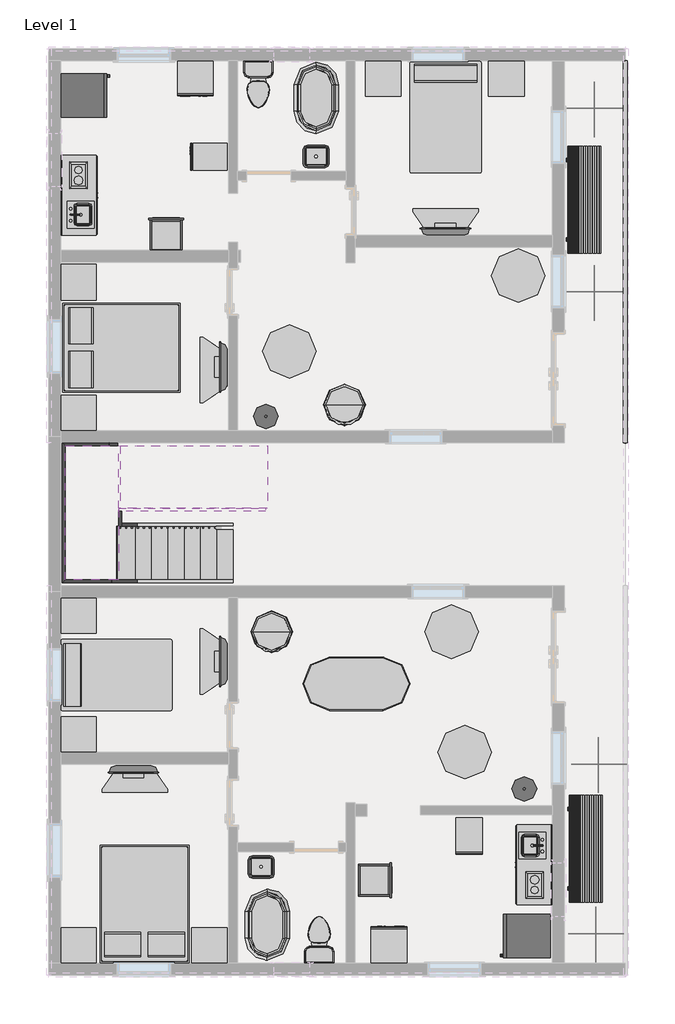
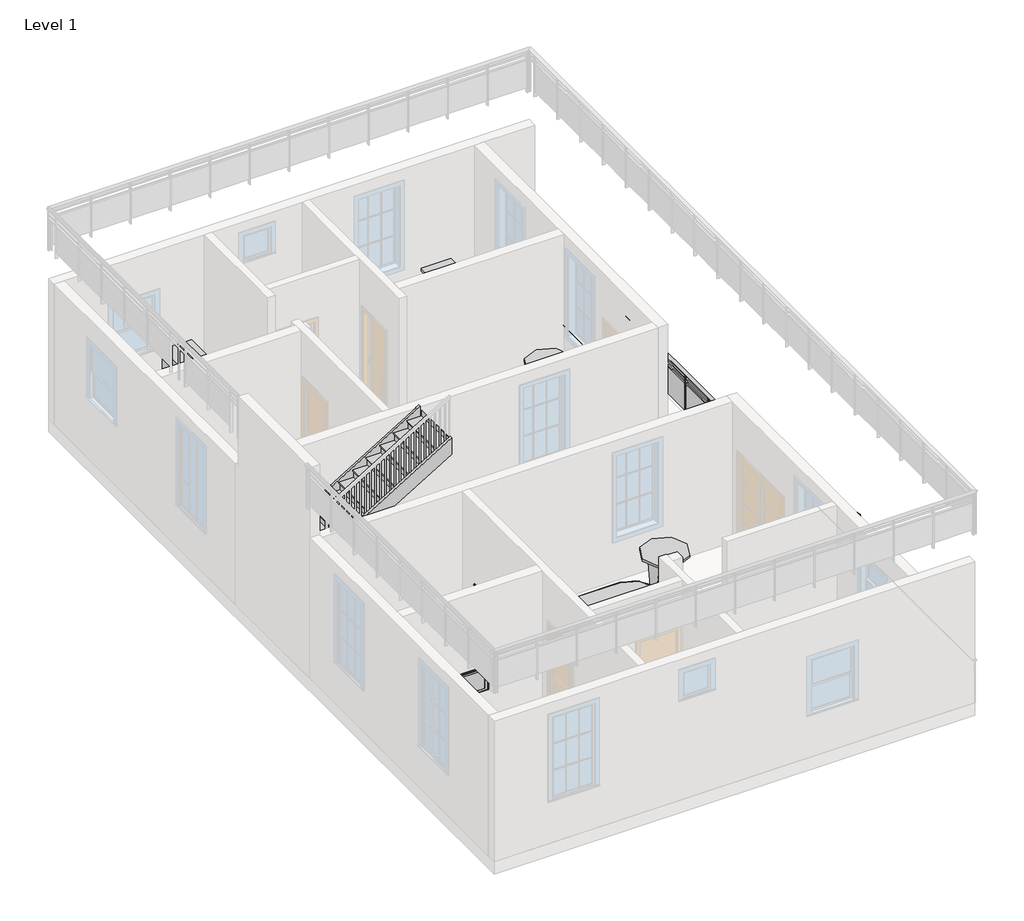
# One storey, part 4 of 4: 29 furniture elements, 12 proxies, 10 flow terminals, 8 members, 6 geographic elements, 2 stair flights, 1 railing, 1 slab.
"""IFC4 building model written with IfcOpenShell, lengths in millimetres."""

from ifc_helpers import new_model, si_unit, point, frame, origin, origin_with_axes, place, context, project, spatial, polyline, ellipse_curve, trimmed, outline, extrude, faceted_brep, transform, mapped, element, save
from ifc_brep_helpers import plane_surface, extruded_surface, advanced_brep
from components import proxy_7e1014cc, proxy_fe84b772, proxy_45b28599, proxy_844211aa, proxy_8b8c2dc4, proxy_a13a33b2, flow_terminal_871c2e40, flow_terminal_d49f872f, flow_terminal_62a433f7, toilet_domestic_3d_toilet_domestic_3d_f7549cf7, toilet_domestic_3d_toilet_domestic_3d_183bbd19, flow_terminal_04541809, furniture_1d2926bd, furniture_4e05012c, furniture_95afb093, furniture_56245f3a, tv_stand_tv_stand_6ce107e5, furniture_2c34a4f9, furniture_905aceb5, furniture_4bee3317, furniture_5bc9ed15, furniture_a7e4c93f, geographic_element_235d1464, rpc_tree_conifer_chinese_juniper_7_1b9786cd, non_monolithic_landing_bbfcd8c5, stair_flight_e984555f, stair_flight_92885a51

model = new_model("IFC4")

# Units and contexts
model_context = context("Model", 3, world=origin())
ifc_project = project(units=[si_unit("LENGTHUNIT", "METRE", prefix="MILLI")], contexts=[model_context])

# Site, building, storey
site = spatial("IfcSite", under=ifc_project)
building = spatial("IfcBuilding", under=site)
storey = spatial("IfcBuildingStorey", under=building, Name="Level 1", Elevation=0.0)

# Proxies
placement = place(None, origin())
proxy_shape = proxy_7e1014cc(model_context)
element("IfcBuildingElementProxy", 1, Name="18\" x 24\" x 34 1/2\"", ObjectType="18\" x 24\" x 34 1/2\"", at=placement, inside=storey, context=model_context, shape_type="MappedRepresentation", body=[
    mapped(proxy_shape, transform((-12093.5246509, 13633.0794856, 0.0), x_axis=(0.0, -0.9999999999999998, 0.0), y_axis=(0.9999999999999998, 0.0, 0.0), z_axis=(0.0, 0.0, 1.0))),
])
element("IfcBuildingElementProxy", 2, Name="18\" x 24\" x 34 1/2\"", ObjectType="18\" x 24\" x 34 1/2\"", at=placement, inside=storey, context=model_context, shape_type="MappedRepresentation", body=[
    mapped(proxy_shape, transform((-7688.1925547, 1465.4124523, 0.0), x_axis=(1.0, 0.0, 0.0), y_axis=(0.0, 1.0, 0.0), z_axis=(0.0, 0.0, 1.0))),
])
proxy_2_shape = proxy_fe84b772(model_context)
element("IfcBuildingElementProxy", 3, Name="Cook Top-2 Unit : 12\" x 18\"", ObjectType="Cook Top-2 Unit : 12\" x 18\"", at=placement, inside=storey, context=model_context, shape_type="MappedRepresentation", body=[
    mapped(proxy_2_shape, transform((-13986.0750862, 13039.6868127, 0.0), x_axis=(-1.0, 0.0, 0.0), y_axis=(0.0, -1.0, 0.0), z_axis=(0.0, 0.0, 1.0))),
])
element("IfcBuildingElementProxy", 4, Name="Cook Top-2 Unit : 12\" x 18\"", ObjectType="Cook Top-2 Unit : 12\" x 18\"", at=placement, inside=storey, context=model_context, shape_type="MappedRepresentation", body=[
    mapped(proxy_2_shape, transform((-6340.6750862, 857.0872215, 0.0), x_axis=(1.0000000000000004, 0.0, 0.0), y_axis=(0.0, 1.0000000000000004, 0.0), z_axis=(0.0, 0.0, 1.0))),
])
proxy_3_shape = proxy_45b28599(model_context)
element("IfcBuildingElementProxy", 5, Name="Dishwasher : 24\" x 24\" x 34\"", ObjectType="Dishwasher : 24\" x 24\" x 34\"", at=placement, inside=storey, context=model_context, shape_type="MappedRepresentation", body=[
    mapped(proxy_3_shape, transform((-12444.3425547, 14419.4124523, 0.0), x_axis=(1.0, 0.0, 0.0), y_axis=(0.0, 1.0, 0.0), z_axis=(0.0, 0.0, 1.0))),
])
element("IfcBuildingElementProxy", 6, Name="Dishwasher : 24\" x 24\" x 34\"", ObjectType="Dishwasher : 24\" x 24\" x 34\"", at=placement, inside=storey, context=model_context, shape_type="MappedRepresentation", body=[
    mapped(proxy_3_shape, transform((-8371.3576177, 118.7115819, 0.0), x_axis=(-1.0000000000000002, 0.0, 0.0), y_axis=(0.0, -1.0000000000000002, 0.0), z_axis=(0.0, 0.0, 1.0))),
])
proxy_4_shape = proxy_844211aa(model_context)
element("IfcBuildingElementProxy", 7, Name="Kitchenette - Small : 54\"", ObjectType="Kitchenette - Small : 54\"", at=placement, inside=storey, context=model_context, shape_type="MappedRepresentation", body=[
    mapped(proxy_4_shape, transform((-14367.0750862, 12647.8243122, 0.0), x_axis=(0.0, 1.0, 0.0), y_axis=(-1.0, 0.0, 0.0), z_axis=(0.0, 0.0, 1.0))),
])
element("IfcBuildingElementProxy", 8, Name="Kitchenette - Small : 54\"", ObjectType="Kitchenette - Small : 54\"", at=placement, inside=storey, context=model_context, shape_type="MappedRepresentation", body=[
    mapped(proxy_4_shape, transform((-5959.6750862, 1248.949722, 0.0), x_axis=(0.0, -1.0000000000000004, 0.0), y_axis=(1.0000000000000004, 0.0, 0.0), z_axis=(0.0, 0.0, 1.0))),
])
proxy_5_shape = proxy_8b8c2dc4(model_context)
element("IfcBuildingElementProxy", 9, Name="Oven Double-Built-in : 21 1/2\" x 39 1/4\" x 21\"", ObjectType="Oven Double-Built-in : 21 1/2\" x 39 1/4\" x 21\"", at=placement, inside=storey, context=model_context, shape_type="MappedRepresentation", body=[
    mapped(proxy_5_shape, transform((-12598.8500135, 12121.827876, 0.0), x_axis=(-1.0000000000000004, 0.0, 0.0), y_axis=(0.0, -1.0000000000000004, 0.0), z_axis=(0.0, 0.0, 1.0))),
])
element("IfcBuildingElementProxy", 10, Name="Oven Double-Built-in : 21 1/2\" x 39 1/4\" x 21\"", ObjectType="Oven Double-Built-in : 21 1/2\" x 39 1/4\" x 21\"", at=placement, inside=storey, context=model_context, shape_type="MappedRepresentation", body=[
    mapped(proxy_5_shape, transform((-8866.6092272, 1005.0369444, 0.0), x_axis=(0.0, 1.0000000000000007, 0.0), y_axis=(-1.0000000000000007, 0.0, 0.0), z_axis=(0.0, 0.0, 1.0))),
])
proxy_6_shape = proxy_a13a33b2(model_context)
element("IfcBuildingElementProxy", 11, Name="Refrigerator : 30\" x 32\" RH", ObjectType="Refrigerator : 30\" x 32\" RH", at=placement, inside=storey, context=model_context, shape_type="MappedRepresentation", body=[
    mapped(proxy_6_shape, transform((-13994.0125862, 14373.5130456, 0.0), x_axis=(0.0, 1.0000000000000002, 0.0), y_axis=(-1.0000000000000002, 0.0, 0.0), z_axis=(0.0, 0.0, 1.0))),
])
element("IfcBuildingElementProxy", 12, Name="Refrigerator : 30\" x 32\" RH", ObjectType="Refrigerator : 30\" x 32\" RH", at=placement, inside=storey, context=model_context, shape_type="MappedRepresentation", body=[
    mapped(proxy_6_shape, transform((-6383.5375862, 12.2109886, 0.0), x_axis=(0.0, -1.0000000000000009, 0.0), y_axis=(1.0000000000000009, 0.0, 0.0), z_axis=(0.0, 0.0, 1.0))),
])

# Flow terminals
flow_terminal_shape = flow_terminal_871c2e40(model_context)
element("IfcFlowTerminal", 13, ObjectType="Sink Kitchen-Island : 18\" x 18\"", at=placement, inside=storey, context=model_context, shape_type="MappedRepresentation", body=[
    mapped(flow_terminal_shape, transform((-14021.829685, 12320.6727765, 0.0), x_axis=(0.0, 1.0, 0.0), y_axis=(-1.0, 0.0, 0.0), z_axis=(0.0, 0.0, 1.0))),
])
element("IfcFlowTerminal", 14, ObjectType="Sink Kitchen-Island : 18\" x 18\"", at=placement, inside=storey, context=model_context, shape_type="MappedRepresentation", body=[
    mapped(flow_terminal_shape, transform((-6304.9204873, 1576.1012577, 0.0), x_axis=(0.0, -1.0000000000000004, 0.0), y_axis=(1.0000000000000004, 0.0, 0.0), z_axis=(0.0, 0.0, 1.0))),
])
flow_terminal_2_shape = flow_terminal_d49f872f(model_context)
element("IfcFlowTerminal", 15, ObjectType="Sink Vanity-Round : 19\" x 19\"", at=placement, inside=storey, context=model_context, shape_type="MappedRepresentation", body=[
    mapped(flow_terminal_2_shape, transform((-6345.6233456, 2611.6039397, 609.6), x_axis=(-1.0000000000000004, 0.0, 0.0), y_axis=(0.0, -1.0000000000000004, 0.0), z_axis=(0.0, 0.0, 1.0))),
])
element("IfcFlowTerminal", 16, ObjectType="Sink Vanity-Round : 19\" x 19\"", at=placement, inside=storey, context=model_context, shape_type="MappedRepresentation", body=[
    mapped(flow_terminal_2_shape, transform((-10762.5691472, 8973.3693513, 609.6), x_axis=(-1.0000000000000004, 0.0, 0.0), y_axis=(0.0, -1.0000000000000004, 0.0), z_axis=(0.0, 0.0, 1.0))),
])
flow_terminal_3_shape = flow_terminal_62a433f7(model_context)
element("IfcFlowTerminal", 17, ObjectType="Sink Vanity-Square : 20\" x 18\"", at=placement, inside=storey, context=model_context, shape_type="MappedRepresentation", body=[
    mapped(flow_terminal_3_shape, transform((-10953.7643267, 1246.916616, 609.6), x_axis=(1.0, 0.0, 0.0), y_axis=(0.0, 1.0, 0.0), z_axis=(0.0, 0.0, 1.0))),
])
element("IfcFlowTerminal", 18, ObjectType="Sink Vanity-Square : 20\" x 18\"", at=placement, inside=storey, context=model_context, shape_type="MappedRepresentation", body=[
    mapped(flow_terminal_3_shape, transform((-9982.5858456, 13278.5074182, 609.6), x_axis=(-1.0000000000000002, 0.0, 0.0), y_axis=(0.0, -1.0000000000000002, 0.0), z_axis=(0.0, 0.0, 1.0))),
])
toilet_domestic_3d_toilet_domestic_3d_shape = toilet_domestic_3d_toilet_domestic_3d_f7549cf7(model_context)
toilet_domestic_3d_toilet_domestic_3d_2_shape = toilet_domestic_3d_toilet_domestic_3d_183bbd19(model_context)
element("IfcFlowTerminal", 19, ObjectType="Toilet-Domestic-3D : Toilet-Domestic-3D", at=placement, inside=storey, context=model_context, shape_type="MappedRepresentation", body=[
    mapped(toilet_domestic_3d_toilet_domestic_3d_shape, transform((-10988.8750862, 14470.5659898, 0.0), x_axis=(1.0, 0.0, 0.0), y_axis=(0.0, 1.0, 0.0), z_axis=(0.0, 0.0, 1.0))),
    mapped(toilet_domestic_3d_toilet_domestic_3d_2_shape, transform((-10988.8750862, 14470.5659898, 0.0), x_axis=(1.0, 0.0, 0.0), y_axis=(0.0, 1.0, 0.0), z_axis=(0.0, 0.0, 1.0))),
])
element("IfcFlowTerminal", 20, ObjectType="Toilet-Domestic-3D : Toilet-Domestic-3D", at=placement, inside=storey, context=model_context, shape_type="MappedRepresentation", body=[
    mapped(toilet_domestic_3d_toilet_domestic_3d_shape, transform((-9947.4750862, 42.1580445, 0.0), x_axis=(-1.0, 0.0, 0.0), y_axis=(0.0, -1.0, 0.0), z_axis=(0.0, 0.0, 1.0))),
    mapped(toilet_domestic_3d_toilet_domestic_3d_2_shape, transform((-9947.4750862, 42.1580445, 0.0), x_axis=(-1.0, 0.0, 0.0), y_axis=(0.0, -1.0, 0.0), z_axis=(0.0, 0.0, 1.0))),
])
flow_terminal_4_shape = flow_terminal_04541809(model_context)
element("IfcFlowTerminal", 21, ObjectType="Tub-Free Standing-3D : 30\" x 60\"", at=placement, inside=storey, context=model_context, shape_type="MappedRepresentation", body=[
    mapped(flow_terminal_4_shape, transform((-10836.4750862, 207.8620171, 0.0), x_axis=(-1.0000000000000004, 0.0, 0.0), y_axis=(0.0, -1.0000000000000004, 0.0), z_axis=(0.0, 0.0, 1.0))),
])
element("IfcFlowTerminal", 22, ObjectType="Tub-Free Standing-3D : 30\" x 60\"", at=placement, inside=storey, context=model_context, shape_type="MappedRepresentation", body=[
    mapped(flow_terminal_4_shape, transform((-9998.2750862, 14330.2620171, 0.0), x_axis=(1.0000000000000002, 0.0, 0.0), y_axis=(0.0, 1.0000000000000002, 0.0), z_axis=(0.0, 0.0, 1.0))),
])

# Furniture
furniture_shape = furniture_1d2926bd(model_context)
element("IfcFurniture", 23, ObjectType="Bed-Box : Queen 60\" x 79\"", at=placement, inside=storey, context=model_context, shape_type="MappedRepresentation", body=[
    mapped(furniture_shape, transform((-12592.8226271, 329.0325089, 0.0), x_axis=(-1.0000000000000004, 0.0, 0.0), y_axis=(0.0, -1.0000000000000004, 0.0), z_axis=(0.0, 0.0, 1.0))),
])
element("IfcFurniture", 24, ObjectType="Bed-Box : Queen 60\" x 79\"", at=placement, inside=storey, context=model_context, shape_type="MappedRepresentation", body=[
    mapped(furniture_shape, transform((-13560.1045944, 9723.9095581, 0.0), x_axis=(0.0, 1.0000000000000002, 0.0), y_axis=(-1.0000000000000002, 0.0, 0.0), z_axis=(0.0, 0.0, 1.0))),
])
furniture_2_shape = furniture_4e05012c(model_context)
element("IfcFurniture", 25, ObjectType="Bed-Standard.0001 : Double 54\" x 75\"", at=placement, inside=storey, context=model_context, shape_type="MappedRepresentation", body=[
    mapped(furniture_2_shape, transform((-13460.1701681, 4203.5734925, 0.0), x_axis=(0.0, 1.0, 0.0), y_axis=(-1.0, 0.0, 0.0), z_axis=(0.0, 0.0, 1.0))),
])
element("IfcFurniture", 26, ObjectType="Bed-Standard.0001 : Double 54\" x 75\"", at=placement, inside=storey, context=model_context, shape_type="MappedRepresentation", body=[
    mapped(furniture_2_shape, transform((-8059.9636108, 14045.6570991, 0.0), x_axis=(1.0000000000000002, 0.0, 0.0), y_axis=(0.0, 1.0000000000000002, 0.0), z_axis=(0.0, 0.0, 1.0))),
])
furniture_3_shape = furniture_95afb093(model_context)
element("IfcFurniture", 27, ObjectType="Counter Top w Sink Hole : 24\" Depth", at=placement, inside=storey, context=model_context, shape_type="MappedRepresentation", body=[
    mapped(furniture_3_shape, transform((-14367.0750862, 13181.2243122, 0.0), x_axis=(0.0, 1.0, 0.0), y_axis=(-1.0, 0.0, 0.0), z_axis=(0.0, 0.0, 1.0))),
])
element("IfcFurniture", 28, ObjectType="Counter Top w Sink Hole : 24\" Depth", at=placement, inside=storey, context=model_context, shape_type="MappedRepresentation", body=[
    mapped(furniture_3_shape, transform((-5959.6750862, 715.549722, 0.0), x_axis=(0.0, -1.0000000000000004, 0.0), y_axis=(1.0000000000000004, 0.0, 0.0), z_axis=(0.0, 0.0, 1.0))),
])
furniture_4_shape = furniture_56245f3a(model_context)
element("IfcFurniture", 29, ObjectType="TV - Flat Screen : 32\"", at=placement, inside=storey, context=model_context, shape_type="MappedRepresentation", body=[
    mapped(furniture_4_shape, transform((-11580.8137098, 9728.917503, 914.4), x_axis=(0.0, -1.0, 0.0), y_axis=(1.0, 0.0, 0.0), z_axis=(0.0, 0.0, 1.0))),
])
element("IfcFurniture", 30, ObjectType="TV - Flat Screen : 32\"", at=placement, inside=storey, context=model_context, shape_type="MappedRepresentation", body=[
    mapped(furniture_4_shape, transform((-7792.4196003, 12039.3006408, 914.4), x_axis=(-1.0, 0.0, 0.0), y_axis=(0.0, -1.0, 0.0), z_axis=(0.0, 0.0, 1.0))),
])
element("IfcFurniture", 31, ObjectType="TV - Flat Screen : 32\"", at=placement, inside=storey, context=model_context, shape_type="MappedRepresentation", body=[
    mapped(furniture_4_shape, transform((-11580.8137098, 4699.717503, 914.4), x_axis=(0.0, -1.0, 0.0), y_axis=(1.0, 0.0, 0.0), z_axis=(0.0, 0.0, 1.0))),
])
element("IfcFurniture", 32, ObjectType="TV - Flat Screen : 32\"", at=placement, inside=storey, context=model_context, shape_type="MappedRepresentation", body=[
    mapped(furniture_4_shape, transform((-13118.530572, 2867.1233935, 914.4), x_axis=(1.0, 0.0, 0.0), y_axis=(0.0, 1.0, 0.0), z_axis=(0.0, 0.0, 1.0))),
])
tv_stand_tv_stand_shape = tv_stand_tv_stand_6ce107e5(model_context)
element("IfcFurniture", 33, ObjectType="TV Stand : TV Stand", at=placement, inside=storey, context=model_context, shape_type="MappedRepresentation", body=[
    mapped(tv_stand_tv_stand_shape, transform((-11522.2750862, 9807.2500192, 0.0), x_axis=(0.0, -1.0, 0.0), y_axis=(1.0, 0.0, 0.0), z_axis=(0.0, 0.0, 1.0))),
])
element("IfcFurniture", 34, ObjectType="TV Stand : TV Stand", at=placement, inside=storey, context=model_context, shape_type="MappedRepresentation", body=[
    mapped(tv_stand_tv_stand_shape, transform((-7663.2870841, 11980.7620171, 0.0), x_axis=(-1.0000000000000004, 0.0, 0.0), y_axis=(0.0, -1.0000000000000004, 0.0), z_axis=(0.0, 0.0, 1.0))),
])
element("IfcFurniture", 35, ObjectType="TV Stand : TV Stand", at=placement, inside=storey, context=model_context, shape_type="MappedRepresentation", body=[
    mapped(tv_stand_tv_stand_shape, transform((-11522.2750862, 4828.8500192, 0.0), x_axis=(0.0, -1.0, 0.0), y_axis=(1.0, 0.0, 0.0), z_axis=(0.0, 0.0, 1.0))),
])
element("IfcFurniture", 36, ObjectType="TV Stand : TV Stand", at=placement, inside=storey, context=model_context, shape_type="MappedRepresentation", body=[
    mapped(tv_stand_tv_stand_shape, transform((-13222.2630882, 2925.6620171, 0.0), x_axis=(1.0000000000000002, 0.0, 0.0), y_axis=(0.0, 1.0000000000000002, 0.0), z_axis=(0.0, 0.0, 1.0))),
])
furniture_5_shape = furniture_2c34a4f9(model_context)
element("IfcFurniture", 37, ObjectType="Table-Dining Oval : 36\" x 72\"", at=placement, inside=storey, context=model_context, shape_type="MappedRepresentation", body=[
    mapped(furniture_5_shape, transform((-8910.655414, 4680.7603778, 0.0), x_axis=(1.0, 0.0, 0.0), y_axis=(0.0, 1.0, 0.0), z_axis=(0.0, 0.0, 1.0))),
])
furniture_6_shape = furniture_905aceb5(model_context)
element("IfcFurniture", 38, ObjectType="Table-Dining Round w Chairs : 36\" Diameter", at=placement, inside=storey, context=model_context, shape_type="MappedRepresentation", body=[
    mapped(furniture_6_shape, transform((-7561.9570534, 3339.1407056, 0.0), x_axis=(1.0, 0.0, 0.0), y_axis=(0.0, 1.0, 0.0), z_axis=(0.0, 0.0, 1.0))),
])
element("IfcFurniture", 39, ObjectType="Table-Dining Round w Chairs : 36\" Diameter", at=placement, inside=storey, context=model_context, shape_type="MappedRepresentation", body=[
    mapped(furniture_6_shape, transform((-10559.1570534, 10184.4407056, 0.0), x_axis=(1.0, 0.0, 0.0), y_axis=(0.0, 1.0, 0.0), z_axis=(0.0, 0.0, 1.0))),
])
furniture_7_shape = furniture_4bee3317(model_context)
element("IfcFurniture", 40, ObjectType="Table-Ellipse : 72\" x 36\"", at=placement, inside=storey, context=model_context, shape_type="MappedRepresentation", body=[
    mapped(furniture_7_shape, transform((-6543.8750862, 11294.9620171, 0.0), x_axis=(1.0, 0.0, 0.0), y_axis=(0.0, 1.0, 0.0), z_axis=(0.0, 0.0, 1.0))),
])
element("IfcFurniture", 41, ObjectType="Table-Ellipse : 72\" x 36\"", at=placement, inside=storey, context=model_context, shape_type="MappedRepresentation", body=[
    mapped(furniture_7_shape, transform((-7686.8750862, 5211.6620171, 0.0), x_axis=(1.0, 0.0, 0.0), y_axis=(0.0, 1.0, 0.0), z_axis=(0.0, 0.0, 1.0))),
])
furniture_8_shape = furniture_5bc9ed15(model_context)
element("IfcFurniture", 42, ObjectType="Table-Night Stand : 24\" x 24\" x 30\"", at=placement, inside=storey, context=model_context, shape_type="MappedRepresentation", body=[
    mapped(furniture_8_shape, transform((-12135.6087165, -452.5379829, 0.0), x_axis=(1.0, 0.0, 0.0), y_axis=(0.0, 1.0, 0.0), z_axis=(0.0, 0.0, 1.0))),
])
element("IfcFurniture", 43, ObjectType="Table-Night Stand : 24\" x 24\" x 30\"", at=placement, inside=storey, context=model_context, shape_type="MappedRepresentation", body=[
    mapped(furniture_8_shape, transform((-14370.8087165, -452.5379829, 0.0), x_axis=(1.0, 0.0, 0.0), y_axis=(0.0, 1.0, 0.0), z_axis=(0.0, 0.0, 1.0))),
])
element("IfcFurniture", 44, ObjectType="Table-Night Stand : 24\" x 24\" x 30\"", at=placement, inside=storey, context=model_context, shape_type="MappedRepresentation", body=[
    mapped(furniture_8_shape, transform((-14370.8087165, 5186.2620171, 0.0), x_axis=(1.0, 0.0, 0.0), y_axis=(0.0, 1.0, 0.0), z_axis=(0.0, 0.0, 1.0))),
])
element("IfcFurniture", 45, ObjectType="Table-Night Stand : 24\" x 24\" x 30\"", at=placement, inside=storey, context=model_context, shape_type="MappedRepresentation", body=[
    mapped(furniture_8_shape, transform((-14370.8087165, 3154.2620171, 0.0), x_axis=(1.0, 0.0, 0.0), y_axis=(0.0, 1.0, 0.0), z_axis=(0.0, 0.0, 1.0))),
])
element("IfcFurniture", 46, ObjectType="Table-Night Stand : 24\" x 24\" x 30\"", at=placement, inside=storey, context=model_context, shape_type="MappedRepresentation", body=[
    mapped(furniture_8_shape, transform((-14370.8087165, 10875.8620171, 0.0), x_axis=(1.0, 0.0, 0.0), y_axis=(0.0, 1.0, 0.0), z_axis=(0.0, 0.0, 1.0))),
])
element("IfcFurniture", 47, ObjectType="Table-Night Stand : 24\" x 24\" x 30\"", at=placement, inside=storey, context=model_context, shape_type="MappedRepresentation", body=[
    mapped(furniture_8_shape, transform((-14370.8087165, 8640.6620171, 0.0), x_axis=(1.0, 0.0, 0.0), y_axis=(0.0, 1.0, 0.0), z_axis=(0.0, 0.0, 1.0))),
])
element("IfcFurniture", 48, ObjectType="Table-Night Stand : 24\" x 24\" x 30\"", at=placement, inside=storey, context=model_context, shape_type="MappedRepresentation", body=[
    mapped(furniture_8_shape, transform((-9163.8087165, 14355.6620171, 0.0), x_axis=(1.0, 0.0, 0.0), y_axis=(0.0, 1.0, 0.0), z_axis=(0.0, 0.0, 1.0))),
])
element("IfcFurniture", 49, ObjectType="Table-Night Stand : 24\" x 24\" x 30\"", at=placement, inside=storey, context=model_context, shape_type="MappedRepresentation", body=[
    mapped(furniture_8_shape, transform((-7055.6087165, 14355.6620171, 0.0), x_axis=(1.0, 0.0, 0.0), y_axis=(0.0, 1.0, 0.0), z_axis=(0.0, 0.0, 1.0))),
])
furniture_9_shape = furniture_a7e4c93f(model_context)
element("IfcFurniture", 50, ObjectType="Table-Round : 36\" Diameter", at=placement, inside=storey, context=model_context, shape_type="MappedRepresentation", body=[
    mapped(furniture_9_shape, transform((-9515.6750862, 9085.1620171, 0.0), x_axis=(1.0, 0.0, 0.0), y_axis=(0.0, 1.0, 0.0), z_axis=(0.0, 0.0, 1.0))),
])
element("IfcFurniture", 51, ObjectType="Table-Round : 36\" Diameter", at=placement, inside=storey, context=model_context, shape_type="MappedRepresentation", body=[
    mapped(furniture_9_shape, transform((-10760.2750862, 5211.6620171, 0.0), x_axis=(1.0, 0.0, 0.0), y_axis=(0.0, 1.0, 0.0), z_axis=(0.0, 0.0, 1.0))),
])

# Geographic elements
geographic_element_shape = geographic_element_235d1464(model_context)
element("IfcGeographicElement", 52, ObjectType="Park Bench : 72\"", at=placement, inside=storey, context=model_context, shape_type="MappedRepresentation", body=[
    mapped(geographic_element_shape, transform((-5426.2750862, 1503.2620171, 0.0), x_axis=(0.0, 1.0000000000000007, 0.0), y_axis=(-1.0000000000000007, 0.0, 0.0), z_axis=(0.0, 0.0, 1.0))),
])
element("IfcGeographicElement", 53, ObjectType="Park Bench : 72\"", at=placement, inside=storey, context=model_context, shape_type="MappedRepresentation", body=[
    mapped(geographic_element_shape, transform((-5451.6750862, 12590.3620171, 0.0), x_axis=(0.0, 1.0000000000000002, 0.0), y_axis=(-1.0000000000000002, 0.0, 0.0), z_axis=(0.0, 0.0, 1.0))),
])
rpc_tree_conifer_chinese_juniper_7_shape = rpc_tree_conifer_chinese_juniper_7_1b9786cd(model_context)
element("IfcGeographicElement", 54, ObjectType="RPC Tree - Conifer : Chinese Juniper - 7'", at=placement, inside=storey, context=model_context, shape_type="MappedRepresentation", body=[
    mapped(rpc_tree_conifer_chinese_juniper_7_shape, transform((-5223.2717572, 55.4620171, 0.0), x_axis=(1.0, 0.0, 0.0), y_axis=(0.0, 1.0, 0.0), z_axis=(0.0, 0.0, 1.0))),
])
element("IfcGeographicElement", 55, ObjectType="RPC Tree - Conifer : Chinese Juniper - 7'", at=placement, inside=storey, context=model_context, shape_type="MappedRepresentation", body=[
    mapped(rpc_tree_conifer_chinese_juniper_7_shape, transform((-5172.4717572, 2951.0620171, 0.0), x_axis=(1.0, 0.0, 0.0), y_axis=(0.0, 1.0, 0.0), z_axis=(0.0, 0.0, 1.0))),
])
element("IfcGeographicElement", 56, ObjectType="RPC Tree - Conifer : Chinese Juniper - 7'", at=placement, inside=storey, context=model_context, shape_type="MappedRepresentation", body=[
    mapped(rpc_tree_conifer_chinese_juniper_7_shape, transform((-5248.6717572, 14152.4620171, 0.0), x_axis=(1.0, 0.0, 0.0), y_axis=(0.0, 1.0, 0.0), z_axis=(0.0, 0.0, 1.0))),
])
element("IfcGeographicElement", 57, ObjectType="RPC Tree - Conifer : Chinese Juniper - 7'", at=placement, inside=storey, context=model_context, shape_type="MappedRepresentation", body=[
    mapped(rpc_tree_conifer_chinese_juniper_7_shape, transform((-5248.6717572, 11015.5620171, 0.0), x_axis=(1.0, 0.0, 0.0), y_axis=(0.0, 1.0, 0.0), z_axis=(0.0, 0.0, 1.0))),
])

# Members
element("IfcMember", 58, ObjectType="Stringer - 2\" Width", at=placement, inside=storey, context=model_context, shape_type="SweptSolid", body=[
    extrude(outline(polyline([(1430.8666667, -13600.7340309), (1126.0666667, -13515.5795744), (2734.3724171, -10861.8750862), (3090.7811786, -10861.8750862), (1430.8666667, -13600.7340309)])), frame((0.0, 8386.6620171, 0.0), z_axis=(0.0, 1.0, 0.0), x_axis=(0.0, 0.0, 1.0)), (0.0, 0.0, 1.0), 50.8),
])
element("IfcMember", 59, ObjectType="Stringer - 2\" Width", at=placement, inside=storey, context=model_context, shape_type="SweptSolid", body=[
    extrude(outline(polyline([(1566.7811786, -13376.4750862), (1210.3724171, -13376.4750862), (2734.3724171, -10861.8750862), (3090.7811786, -10861.8750862), (1566.7811786, -13376.4750862)])), frame((0.0, 7269.0620171, 0.0), z_axis=(0.0, 1.0, 0.0), x_axis=(0.0, 0.0, 1.0)), (0.0, 0.0, 1.0), 50.8),
])
element("IfcMember", 60, ObjectType="Stringer - 2\" Width", at=placement, inside=storey, context=model_context, shape_type="SweptSolid", body=[
    extrude(outline(polyline([(0.0, -11420.6750862), (212.114512, -11420.6750862), (1430.8666667, -13431.6161414), (1126.0666667, -13516.7705979), (0.0, -11658.7605979), (0.0, -11420.6750862)])), frame((0.0, 6049.8620171, 0.0), z_axis=(0.0, 1.0, 0.0), x_axis=(0.0, 0.0, 1.0)), (0.0, 0.0, 1.0), 50.8),
])
element("IfcMember", 61, ObjectType="Stringer - 2\" Width", at=placement, inside=storey, context=model_context, shape_type="SweptSolid", body=[
    extrude(outline(polyline([(0.0, -11420.6750862), (212.114512, -11420.6750862), (1366.6599665, -13325.6750862), (1010.251205, -13325.6750862), (0.0, -11658.7605979), (0.0, -11420.6750862)])), frame((0.0, 7015.0620171, 0.0), z_axis=(0.0, 1.0, 0.0), x_axis=(0.0, 0.0, 1.0)), (0.0, 0.0, 1.0), 50.8),
])
element("IfcMember", 62, ObjectType="Stringer - 2\" Width", at=placement, inside=storey, context=model_context, shape_type="Brep", body=[
    faceted_brep([(-13600.7340309, 8386.6620171, 1430.8666667), (-13600.7340309, 8437.4620171, 1430.8666667), (-14341.6750862, 8437.4620171, 1430.8666667), (-14290.8750862, 8386.6620171, 1430.8666667), (-13515.5795744, 8386.6620171, 1126.0666667), (-14290.8750862, 8386.6620171, 1126.0666667), (-13515.5795744, 8437.4620171, 1126.0666667), (-14341.6750862, 8437.4620171, 1126.0666667)], [[[0, 1, 2, 3]], [[4, 0, 3, 5]], [[6, 4, 5, 7]], [[1, 6, 7, 2]], [[1, 0, 4, 6]], [[2, 7, 5, 3]]]),
])
element("IfcMember", 63, ObjectType="Stringer - 2\" Width", at=placement, inside=storey, context=model_context, shape_type="SweptSolid", body=[
    extrude(outline(polyline([(-14341.6750862, 8437.4620171), (-14290.8750862, 8386.6620171), (-14290.8750862, 6100.6620171), (-14341.6750862, 6049.8620171), (-14341.6750862, 8437.4620171)])), frame((0.0, 0.0, 1126.0666667), z_axis=(0.0, 0.0, 1.0), x_axis=(1.0, 0.0, 0.0)), (0.0, 0.0, 1.0), 304.8),
])
element("IfcMember", 64, ObjectType="Stringer - 2\" Width", at=placement, inside=storey, context=model_context, shape_type="Brep", body=[
    faceted_brep([(-14290.8750862, 6100.6620171, 1430.8666667), (-14341.6750862, 6049.8620171, 1430.8666667), (-13431.6161414, 6049.8620171, 1430.8666667), (-13431.6161414, 6100.6620171, 1430.8666667), (-14290.8750862, 6100.6620171, 1126.0666667), (-13516.7705979, 6100.6620171, 1126.0666667), (-14341.6750862, 6049.8620171, 1126.0666667), (-13516.7705979, 6049.8620171, 1126.0666667)], [[[0, 1, 2, 3]], [[4, 0, 3, 5]], [[6, 4, 5, 7]], [[1, 6, 7, 2]], [[1, 0, 4, 6]], [[2, 7, 5, 3]]]),
])
element("IfcMember", 65, ObjectType="Stringer - 2\" Width", at=placement, inside=storey, context=model_context, shape_type="SweptSolid", body=[
    extrude(outline(polyline([(-13325.6750862, 7015.0620171), (-13376.4750862, 7015.0620171), (-13376.4750862, 7269.0620171), (-13325.6750862, 7269.0620171), (-13325.6750862, 7015.0620171)])), frame((0.0, 0.0, 1126.0666667), z_axis=(0.0, 0.0, 1.0), x_axis=(1.0, 0.0, 0.0)), (0.0, 0.0, 1.0), 304.8),
])

# Railing
element("IfcRailing", 66, ObjectType="Glass Panel - Bottom Fill", at=placement, inside=storey, context=model_context, shape_type="SolidModel", body=[
    advanced_brep(
    [(-4753.1750862, 8437.4620171, 914.4), (-4676.9750862, 8437.4620171, 914.4), (-4753.1750862, 14965.2620171, 914.4), (-4676.9750862, 14965.2620171, 914.4)],
    [
        (0, 1, ellipse_curve(frame((-4715.0750862, 8437.4620171, 914.4), z_axis=(0.0, -1.0, 0.0), x_axis=(1.0, 0.0, 0.0)), 38.1, 28.575)),
        (1, 0, ellipse_curve(frame((-4715.0750862, 8437.4620171, 914.4), z_axis=(0.0, -1.0, 0.0), x_axis=(1.0, 0.0, 0.0)), 38.1, 28.575)),
        (2, 3, ellipse_curve(frame((-4715.0750862, 14965.2620171, 914.4), z_axis=(0.0, 1.0, 0.0), x_axis=(1.0, 0.0, 0.0)), 38.1, 28.575)),
        (3, 2, ellipse_curve(frame((-4715.0750862, 14965.2620171, 914.4), z_axis=(0.0, 1.0, 0.0), x_axis=(1.0, 0.0, 0.0)), 38.1, 28.575)),
        (0, 2),
        (3, 1),
    ],
    [
        plane_surface(frame((-4715.0750862, 8437.4620171, 914.4), z_axis=(0.0, -1.0, 0.0), x_axis=(0.0, 0.0, 1.0))),
        plane_surface(frame((-4715.0750862, 14965.2620171, 914.4), z_axis=(0.0, 1.0, 0.0), x_axis=(0.0, 0.0, 1.0))),
        extruded_surface(trimmed(ellipse_curve(frame((-4715.0750862, 14965.2620171, 914.4), z_axis=(0.0, -1.0, 0.0), x_axis=(1.0, 0.0, 0.0)), 38.1, 28.575), [point((-4753.1750862, 14965.2620171, 914.4))], [point((-4676.9750862, 14965.2620171, 914.4))], True, "CARTESIAN"), (0.0, -6527.799999999999, 0.0), 6527.799999999999),
        extruded_surface(trimmed(ellipse_curve(frame((-4715.0750862, 14965.2620171, 914.4), z_axis=(0.0, -1.0, 0.0), x_axis=(1.0, 0.0, 0.0)), 38.1, 28.575), [point((-4676.9750862, 14965.2620171, 914.4))], [point((-4753.1750862, 14965.2620171, 914.4))], True, "CARTESIAN"), (0.0, -6527.799999999999, 0.0), 6527.799999999999),
    ],
    [
        (0, [[1, 2]]),
        (1, [[3, 4]]),
        (2, [[-1, 5, -4, 6]]),
        (3, [[-2, -6, -3, -5]]),
    ],
),
    extrude(outline(polyline([(-4702.3750862, 8437.4620171), (-4727.7750862, 8437.4620171), (-4727.7750862, 14965.2620171), (-4702.3750862, 14965.2620171), (-4702.3750862, 8437.4620171)])), frame((0.0, 0.0, 800.1), z_axis=(0.0, 0.0, 1.0), x_axis=(1.0, 0.0, 0.0)), (0.0, 0.0, 1.0), 25.4),
    extrude(outline(polyline([(-4702.3750862, 8437.4620171), (-4727.7750862, 8437.4620171), (-4727.7750862, 14965.2620171), (-4702.3750862, 14965.2620171), (-4702.3750862, 8437.4620171)])), frame((0.0, 0.0, 698.5), z_axis=(0.0, 0.0, 1.0), x_axis=(1.0, 0.0, 0.0)), (0.0, 0.0, 1.0), 25.4),
    extrude(outline(polyline([(-4689.6750862, 14463.6120171), (-4740.4750862, 14463.6120171), (-4740.4750862, 14476.3120171), (-4689.6750862, 14476.3120171), (-4689.6750862, 14463.6120171)])), origin_with_axes(), (0.0, 0.0, 1.0), 885.6788223),
    extrude(outline(polyline([(-4721.6102432, 13657.1620171), (-4721.6102432, 14469.9620171), (-4715.2602432, 14469.9620171), (-4715.2602432, 13657.1620171), (-4721.6102432, 13657.1620171)])), frame((0.0, 0.0, 101.6), z_axis=(0.0, 0.0, 1.0), x_axis=(1.0, 0.0, 0.0)), (0.0, 0.0, 1.0), 596.9),
    extrude(outline(polyline([(-4689.6750862, 13650.8120171), (-4740.4750862, 13650.8120171), (-4740.4750862, 13663.5120171), (-4689.6750862, 13663.5120171), (-4689.6750862, 13650.8120171)])), origin_with_axes(), (0.0, 0.0, 1.0), 885.6788223),
    extrude(outline(polyline([(-4721.6102432, 12844.3620171), (-4721.6102432, 13657.1620171), (-4715.2602432, 13657.1620171), (-4715.2602432, 12844.3620171), (-4721.6102432, 12844.3620171)])), frame((0.0, 0.0, 101.6), z_axis=(0.0, 0.0, 1.0), x_axis=(1.0, 0.0, 0.0)), (0.0, 0.0, 1.0), 596.9),
    extrude(outline(polyline([(-4689.6750862, 12838.0120171), (-4740.4750862, 12838.0120171), (-4740.4750862, 12850.7120171), (-4689.6750862, 12850.7120171), (-4689.6750862, 12838.0120171)])), origin_with_axes(), (0.0, 0.0, 1.0), 885.6788223),
    extrude(outline(polyline([(-4721.6102432, 12031.5620171), (-4721.6102432, 12844.3620171), (-4715.2602432, 12844.3620171), (-4715.2602432, 12031.5620171), (-4721.6102432, 12031.5620171)])), frame((0.0, 0.0, 101.6), z_axis=(0.0, 0.0, 1.0), x_axis=(1.0, 0.0, 0.0)), (0.0, 0.0, 1.0), 596.9),
    extrude(outline(polyline([(-4689.6750862, 12025.2120171), (-4740.4750862, 12025.2120171), (-4740.4750862, 12037.9120171), (-4689.6750862, 12037.9120171), (-4689.6750862, 12025.2120171)])), origin_with_axes(), (0.0, 0.0, 1.0), 885.6788223),
    extrude(outline(polyline([(-4721.6102432, 11218.7620171), (-4721.6102432, 12031.5620171), (-4715.2602432, 12031.5620171), (-4715.2602432, 11218.7620171), (-4721.6102432, 11218.7620171)])), frame((0.0, 0.0, 101.6), z_axis=(0.0, 0.0, 1.0), x_axis=(1.0, 0.0, 0.0)), (0.0, 0.0, 1.0), 596.9),
    extrude(outline(polyline([(-4689.6750862, 11212.4120171), (-4740.4750862, 11212.4120171), (-4740.4750862, 11225.1120171), (-4689.6750862, 11225.1120171), (-4689.6750862, 11212.4120171)])), origin_with_axes(), (0.0, 0.0, 1.0), 885.6788223),
    extrude(outline(polyline([(-4721.6102432, 10405.9620171), (-4721.6102432, 11218.7620171), (-4715.2602432, 11218.7620171), (-4715.2602432, 10405.9620171), (-4721.6102432, 10405.9620171)])), frame((0.0, 0.0, 101.6), z_axis=(0.0, 0.0, 1.0), x_axis=(1.0, 0.0, 0.0)), (0.0, 0.0, 1.0), 596.9),
    extrude(outline(polyline([(-4689.6750862, 10399.6120171), (-4740.4750862, 10399.6120171), (-4740.4750862, 10412.3120171), (-4689.6750862, 10412.3120171), (-4689.6750862, 10399.6120171)])), origin_with_axes(), (0.0, 0.0, 1.0), 885.6788223),
    extrude(outline(polyline([(-4721.6102432, 9593.1620171), (-4721.6102432, 10405.9620171), (-4715.2602432, 10405.9620171), (-4715.2602432, 9593.1620171), (-4721.6102432, 9593.1620171)])), frame((0.0, 0.0, 101.6), z_axis=(0.0, 0.0, 1.0), x_axis=(1.0, 0.0, 0.0)), (0.0, 0.0, 1.0), 596.9),
    extrude(outline(polyline([(-4689.6750862, 9586.8120171), (-4740.4750862, 9586.8120171), (-4740.4750862, 9599.5120171), (-4689.6750862, 9599.5120171), (-4689.6750862, 9586.8120171)])), origin_with_axes(), (0.0, 0.0, 1.0), 885.6788223),
    extrude(outline(polyline([(-4721.6102432, 8780.3620171), (-4721.6102432, 9593.1620171), (-4715.2602432, 9593.1620171), (-4715.2602432, 8780.3620171), (-4721.6102432, 8780.3620171)])), frame((0.0, 0.0, 101.6), z_axis=(0.0, 0.0, 1.0), x_axis=(1.0, 0.0, 0.0)), (0.0, 0.0, 1.0), 596.9),
    extrude(outline(polyline([(-4689.6750862, 8774.0120171), (-4740.4750862, 8774.0120171), (-4740.4750862, 8786.7120171), (-4689.6750862, 8786.7120171), (-4689.6750862, 8774.0120171)])), origin_with_axes(), (0.0, 0.0, 1.0), 885.6788223),
    extrude(outline(polyline([(-4705.5500862, 14803.3370171), (-4724.6000862, 14803.3370171), (-4724.6000862, 14822.3870171), (-4705.5500862, 14822.3870171), (-4705.5500862, 14803.3370171)])), origin_with_axes(), (0.0, 0.0, 1.0), 885.6788223),
    extrude(outline(polyline([(-4705.5500862, 14952.5620171), (-4724.6000862, 14952.5620171), (-4724.6000862, 14971.6120171), (-4705.5500862, 14971.6120171), (-4705.5500862, 14952.5620171)])), origin_with_axes(), (0.0, 0.0, 1.0), 885.6788223),
    extrude(outline(polyline([(-4705.5500862, 8431.1120171), (-4724.6000862, 8431.1120171), (-4724.6000862, 8450.1620171), (-4705.5500862, 8450.1620171), (-4705.5500862, 8431.1120171)])), origin_with_axes(), (0.0, 0.0, 1.0), 885.6788223),
])

# Slab
non_monolithic_landing_shape = non_monolithic_landing_bbfcd8c5(model_context)
element("IfcSlab", 67, ObjectType="Non-Monolithic Landing", at=placement, inside=storey, context=model_context, shape_type="MappedRepresentation", body=[
    mapped(non_monolithic_landing_shape, transform((0.0, 0.0, 0.0), x_axis=(1.0, 0.0, 0.0), y_axis=(0.0, 1.0, 0.0), z_axis=(0.0, 0.0, 1.0))),
])

# Stair flights
stair_flight_shape = stair_flight_e984555f(model_context)
element("IfcStairFlight", 68, ObjectType="2\" Tread 1\" Nosing 1/4\" Riser", at=placement, inside=storey, context=model_context, shape_type="MappedRepresentation", body=[
    mapped(stair_flight_shape, transform((0.0, 0.0, 0.0), x_axis=(1.0, 0.0, 0.0), y_axis=(0.0, 1.0, 0.0), z_axis=(0.0, 0.0, 1.0))),
])
stair_flight_2_shape = stair_flight_92885a51(model_context)
element("IfcStairFlight", 69, ObjectType="2\" Tread 1\" Nosing 1/4\" Riser", at=placement, inside=storey, context=model_context, shape_type="MappedRepresentation", body=[
    mapped(stair_flight_2_shape, transform((0.0, 0.0, 0.0), x_axis=(1.0, 0.0, 0.0), y_axis=(0.0, 1.0, 0.0), z_axis=(0.0, 0.0, 1.0))),
])

save(model, "model.ifc")

# Revit data of these elements
# Type "18\" x 24\" x 34 1/2\""
#   Label = "T"
#   Assembly Code = "E1090400"
#   Depth = 2' - 0"
#   Height = 2' - 10 1/2"
#   Width = 1' - 6"
#   Panel Face Material = Plastic, Opaque Black
#   Trach Compact. Material = Steel, Paint Finish, Ivory, Matte
#   Default Elevation = 0
# Type "Cook Top-2 Unit : 12\" x 18\""
#   Assembly Code = "E1090400"
#   Counter Height = 3' - 0"
#   Depth = 1' - 6"
#   Width = 1' - 0"
#   Burner Material = Steel, Chrome Plated
#   Cooktop Material = Steel, Polished
#   Default Elevation = 0
# Type "Dishwasher : 24\" x 24\" x 34\""
#   Label = "DW"
#   Assembly Code = "E1090400"
#   Depth = 2' - 0"
#   Height = 2' - 10"
#   Width = 2' - 0"
#   Dishwasher Material = Steel, Paint Finish, Ivory, Glossy
#   Panel Face Material = Plastic, Opaque Black
#   Default Elevation = 0
# Type "Kitchenette - Small : 54\""
#   Assembly Code = "E1090400"
#   Width = 4' - 6"
#   Height = 2' - 10 1/2"
#   Depth = 2' - 0"
#   Toe Depth = 0' - 3"
#   Toe Height = 0' - 3 1/2"
#   Cabinet Material = Cabinets
#   Door/Drawer Material = Cabinets
#   Handle Material = Cabinets - Handles
#   Default Elevation = 0
# Type "Oven Double-Built-in : 21 1/2\" x 39 1/4\" x 21\""
#   Label = "OVEN"
#   Assembly Code = "E1090400"
#   Depth = 1' - 9"
#   Height = 3' - 3 1/4"
#   Width = 1' - 9 1/2"
#   Oven Material = Metal - Stainless Steel, Polished
#   Default Elevation = 0
# Type "Refrigerator : 30\" x 32\" RH"
#   Label = "REF."
#   Assembly Code = "E1090400"
#   Depth = 2' - 7 3/4"
#   Handle = 2' - 3"
#   Height = 5' - 10"
#   Rear Clearance = 0' - 2"
#   Top Door Height = 1' - 8"
#   Width = 2' - 5 3/8"
#   Material = Steel, Paint Finish, Ivory, Glossy
#   Default Elevation = 0
# Type "Sink Kitchen-Island : 18\" x 18\""
#   Assembly Code = "D2010410"
#   Counter Height = 3' - 0"
#   Depth = 1' - 6"
#   Width = 1' - 6"
#   Faucet Material = Steel, Polished
#   Sink Material = Steel, Polished
#   Default Elevation = 0
# Type "Sink Vanity-Round : 19\" x 19\""
#   Assembly Code = "D2010400"
#   Top Of Counter = 2' - 7"
#   Basin Material = Porcelain, Linen
#   Faucet Material = Steel, Polished
#   Default Elevation = 0
# Type "Sink Vanity-Square : 20\" x 18\""
#   Assembly Code = "D2010400"
#   Counter Height = 2' - 7"
#   Depth = 1' - 6"
#   Width = 1' - 8"
#   Basin Material = Porcelain, Linen
#   Faucet Material = Steel, Polished
#   Default Elevation = 0
# Type "Toilet-Domestic-3D : Toilet-Domestic-3D"
#   Assembly Code = "D2010110"
#   Toilet - Bowl/Basin Material = Porcelain, Linen
#   Toilet - Seat Material = Laminate, Linen, Matte
#   Default Elevation = 0
# Type "Tub-Free Standing-3D : 30\" x 60\""
#   Assembly Code = "D2010110"
#   Height = 1' - 6"
#   Length = 4' - 0"
#   Width = 2' - 6"
#   Tub Material = Porcelain, Ivory
#   Default Elevation = 0
# Type "Bed-Box : Queen 60\" x 79\""
#   Assembly Code = "E2020200"
#   Length = 6' - 7"
#   Width = 5' - 0"
#   Frame Material = Birch
#   Mattress Material = Linen, White
#   Default Elevation = 0
# Type "Bed-Standard.0001 : Double 54\" x 75\""
#   Assembly Code = "E2020200"
#   Length = 6' - 3"
#   Width = 4' - 0"
#   Leg Material = Steel, Chrome Plated
#   Mattress Material = Linen, White
#   Default Elevation = 0
# Type "Counter Top w Sink Hole : 24\" Depth"
#   Assembly Code = "C1030400"
#   Counter Thickness = 0' - 1 1/2"
#   Depth [instance default] = 2' - 1"
#   Height = 3' - 0"
#   Length [instance default] = 8' - 0"
#   Sink Location [instance default] = 2' - 0"
#   Sink Location To Wall [instance default] = 0' - 6"
#   Sink Opening Depth [instance default] = 1' - 3"
#   Sink Opening Width [instance default] = 2' - 3"
#   Counter Top Material = none
#   Default Elevation = 0
# Type "TV - Flat Screen : 32\""
#   SinAng = 0' - 0.0193"
#   L = 2' - 3.79372"
#   H = 1' - 3.6354"
#   Thickness = 0' - 4.33071"
#   Diagonal = 2' - 7.88976"
#   CosAng = 0' - 0.03431"
#   Stand [instance default] = yes
#   Default Elevation = 0
# Type "TV Stand : TV Stand"
#   Depth = 1' - 6"
#   Width = 3' - 8"
#   Height = 1' - 7 1/2"
#   Finish = Melamine - Gray
#   Default Elevation = 0
# Type "Table-Dining Oval : 36\" x 72\""
#   Assembly Code = "E2020200"
#   Length = 6' - 0"
#   Width = 3' - 0"
#   Base Material = Steel, Chrome Plated
#   Top Material = Glass - Clear, Grey
#   Default Elevation = 0
#   Description = (empty or 0)
# Type "Table-Dining Round w Chairs : 36\" Diameter"
#   Assembly Code = "E2020200"
#   Radius = 1' - 6"
#   Diameter = 3' - 0"
#   Height = 2' - 6"
#   Chairs = 4
#   Base Material = Pine
#   Top Material = Laminate, Linen, Matte
#   Default Elevation = 0
# Type "Table-Ellipse : 72\" x 36\""
#   Assembly Code = "E2020200"
#   Half Width = 1' - 6"
#   Half Length = 1' - 6"
#   Height = 2' - 6"
#   Length = 3' - 0"
#   Width = 3' - 0"
#   Base Material = Birch
#   Top Material = Laminate - Black
#   Default Elevation = 0
# Type "Table-Night Stand : 24\" x 24\" x 30\""
#   Assembly Code = "E2020200"
#   Depth = 2' - 0"
#   Height = 2' - 6"
#   Width = 2' - 0"
#   Base Material = Birch
#   Top Material = Laminate, Ivory, Matte
#   Default Elevation = 0
# Type "Table-Round : 36\" Diameter"
#   Assembly Code = "E2020200"
#   Base Radius = 0' - 10"
#   Height = 2' - 6"
#   Radius = 1' - 2"
#   Base Material = Steel, Chrome Plated
#   Top Material = Birch
#   Default Elevation = 0
# Type "Park Bench : 72\""
#   Length = 6' - 0"
#   Seat Material = Wood - Teak
#   Frame Material = Steel, Paint Finish, Dark Gray, Matte
# Type "RPC Tree - Conifer : Chinese Juniper - 7'"
#   built-in parameter 1005198 = "{2, 15},{39, RPC-16-FUM3-UUQ0-UBF0-N000-ST1L-LVER-AU},{1, 0},{1, 0},{2, 13},{1, 8},{5, Color},{1, 0},{1, 0},{3, 0.8},{3, 0.8},{3, 0.8},{1, 8},{7, BBoxMin},{1, 0},{1, 0},{1, 0},{1, 0},{1, 0},{1, 8},{7, BBoxMax},{1, 0},{1, 0},{1, 0},{1, 0},{1, 0},{2, 11},{9, RPCTypeId},{1, 0},{1, 0},{39, RPC-16-FUM3-UUQ0-UBF0-N000-ST1L-LVER-AU},{1, 6},{14, RPCPlantHeight},{1, 0},{1, 0},{1, 7},{2, 11},{7, keyword},{1, 0},{1, 0},{34, :RPCs:Trees [General]:Geometry:RPC},{2, 11},{8, category},{1, 0},{1, 0},{15, Trees [General]},{2, 11},{12, LocalizedUID},{1, 0},{1, 0},{15, Chinese Juniper},{2, 14},{6, Height},{1, 0},{1, 0},{1, 7},{1, 2},{16, Cast Reflections},{1, 0},{1, 0},{1, 0},{1, 2},{12, Cast Shadows},{1, 0},{1, 0},{1, 1},{1, 2},{9, Lock View},{1, 0},{1, 0},{1, 0},{1, 4},{5, ViewC},{1, 0},{1, 0},{1, 0},{21, assetlibrary_base.fbx},{1, 5},"
#   built-in parameter 1005195 = "RPC-16-FUM3-UUQ0-UBF0-N000-ST1L-LVER-AU"
#   Type Comments = "Chinese Juniper"
#   Assembly Code = "G2050500"
#   Height = 7' - 0"
#   Description = (empty or 0)
#   Default Elevation = 0
# Type "Glass Panel - Bottom Fill"
#   Assembly Code = "C2010400"
#   built-in parameter 1008612 = 0.0416667 (stored number, unit not read)
#   built-in parameter 1008611 = 0.0416667 (stored number, unit not read)
#   built-in parameter 1008609 = 0.333333 (stored number, unit not read)
#   built-in parameter 1008604 = 0.166667 (stored number, unit not read)
#   built-in parameter 1008603 = 0.166667 (stored number, unit not read)
#   Railing Height = 3' - 0"
#   built-in parameter 1008630 = 2
#   built-in parameter 1008610 = 2
#   built-in parameter 1008618 = Baluster - Square : 3/4"
# Elements 1, 2 (IfcBuildingElementProxy, "18\" x 24\" x 34 1/2\"")
#   Phase Created = New Construction
#   Materials on its faces: "Steel, Paint Finish, Ivory, Matte", "Plastic, Opaque Black"
# Elements 3, 4 (IfcBuildingElementProxy, "Cook Top-2 Unit : 12\" x 18\"")
#   Phase Created = New Construction
#   Materials on its faces: "Steel, Chrome Plated", "Steel, Polished"
# Elements 5, 6 (IfcBuildingElementProxy, "Dishwasher : 24\" x 24\" x 34\"")
#   Phase Created = New Construction
#   Materials on its faces: "Steel, Paint Finish, Ivory, Glossy", "Plastic, Opaque Black"
# Elements 7, 8 (IfcBuildingElementProxy, "Kitchenette - Small : 54\"")
#   Phase Created = New Construction
#   Materials on its faces: "Cabinets", "Cabinets - Handles"
# Elements 9, 10 (IfcBuildingElementProxy, "Oven Double-Built-in : 21 1/2\" x 39 1/4\" x 21\"")
#   Phase Created = New Construction
#   Materials on its faces: "Steel", "Metal - Stainless Steel, Polished", "Glass"
# Elements 11, 12 (IfcBuildingElementProxy, "Refrigerator : 30\" x 32\" RH")
#   Phase Created = New Construction
#   Materials on its faces: "Steel, Paint Finish, Ivory, Glossy", "Steel, Chrome Plated"
# Element 13 (IfcFlowTerminal, "Sink Kitchen-Island : 18\" x 18\"")
#   Mark = "7"
#   Phase Created = New Construction
#   Materials on its faces: "Steel, Polished"
# Element 14 (IfcFlowTerminal, "Sink Kitchen-Island : 18\" x 18\"")
#   Mark = "9"
#   Phase Created = New Construction
#   Materials on its faces: "Steel, Polished"
# Element 15 (IfcFlowTerminal, "Sink Vanity-Round : 19\" x 19\"")
#   Mark = "10"
#   Phase Created = New Construction
#   Materials on its faces: "Porcelain, Linen", "Steel, Polished"
# Element 16 (IfcFlowTerminal, "Sink Vanity-Round : 19\" x 19\"")
#   Mark = "11"
#   Phase Created = New Construction
#   Materials on its faces: "Porcelain, Linen", "Steel, Polished"
# Element 17 (IfcFlowTerminal, "Sink Vanity-Square : 20\" x 18\"")
#   Mark = "5"
#   Phase Created = New Construction
#   Materials on its faces: "Porcelain, Linen", "Steel, Polished"
# Element 18 (IfcFlowTerminal, "Sink Vanity-Square : 20\" x 18\"")
#   Mark = "6"
#   Phase Created = New Construction
#   Materials on its faces: "Porcelain, Linen", "Steel, Polished"
# Element 19 (IfcFlowTerminal, "Toilet-Domestic-3D : Toilet-Domestic-3D")
#   Mark = "1"
#   Phase Created = New Construction
#   Materials on its faces: "Porcelain, Linen", "Laminate, Linen, Matte"
# Element 20 (IfcFlowTerminal, "Toilet-Domestic-3D : Toilet-Domestic-3D")
#   Mark = "2"
#   Phase Created = New Construction
#   Materials on its faces: "Porcelain, Linen", "Laminate, Linen, Matte"
# Element 21 (IfcFlowTerminal, "Tub-Free Standing-3D : 30\" x 60\"")
#   Mark = "3"
#   Phase Created = New Construction
#   Materials on its faces: "Porcelain, Ivory"
# Element 22 (IfcFlowTerminal, "Tub-Free Standing-3D : 30\" x 60\"")
#   Mark = "4"
#   Phase Created = New Construction
#   Materials on its faces: "Porcelain, Ivory"
# Elements 23, 24 (IfcFurniture, "Bed-Box : Queen 60\" x 79\"")
#   Phase Created = New Construction
#   Materials on its faces: "Birch", "Linen, White"
# Elements 25, 26 (IfcFurniture, "Bed-Standard.0001 : Double 54\" x 75\"")
#   Phase Created = New Construction
#   Materials on its faces: "Linen, White", "Steel, Chrome Plated"
# Elements 27, 28 (IfcFurniture, "Counter Top w Sink Hole : 24\" Depth")
#   Sink Opening Depth = 1' - 3"
#   Sink Location To Wall = 0' - 6"
#   Length = 4' - 6"
#   Sink Location = 1' - 2"
#   Sink Opening Width = 1' - 4"
#   Depth = 2' - 0"
#   Phase Created = New Construction
#   Materials on its faces: "Counter Top"
# Elements 29, 30, 31, 32 (IfcFurniture, "TV - Flat Screen : 32\"")
#   Stand = yes
#   Phase Created = New Construction
#   Materials on its faces: "TV - Black", "TV - Glass", "TV - Screen"
# Elements 33, 34, 35, 36 (IfcFurniture, "TV Stand : TV Stand")
#   Phase Created = New Construction
#   Materials on its faces: "Melamine - Gray", "Glass - Shelves"
# Element 37 (IfcFurniture, "Table-Dining Oval : 36\" x 72\"")
#   Phase Created = New Construction
#   Materials on its faces: "Steel, Chrome Plated", "Glass - Clear, Grey"
# Elements 38, 39 (IfcFurniture, "Table-Dining Round w Chairs : 36\" Diameter")
#   Phase Created = New Construction
#   Materials on its faces: "Pine", "Laminate, Linen, Matte"
# Elements 40, 41 (IfcFurniture, "Table-Ellipse : 72\" x 36\"")
#   Phase Created = New Construction
#   Materials on its faces: "Birch", "Laminate - Black"
# Elements 42, 43, 44, 45, 46, 47, 48, 49 (IfcFurniture, "Table-Night Stand : 24\" x 24\" x 30\"")
#   Phase Created = New Construction
#   Materials on its faces: "Birch", "Laminate, Ivory, Matte"
# Elements 50, 51 (IfcFurniture, "Table-Round : 36\" Diameter")
#   Phase Created = New Construction
#   Materials on its faces: "Steel, Chrome Plated", "Birch"
# Elements 52, 53 (IfcGeographicElement, "Park Bench : 72\"")
#   Phase Created = New Construction
#   Materials on its faces: "Wood - Teak", "Steel, Paint Finish, Dark Gray, Matte"
# Elements 54, 55, 56, 57 (IfcGeographicElement, "RPC Tree - Conifer : Chinese Juniper - 7'")
#   Phase Created = New Construction
# Elements 58, 59, 60, 61, 62, 63, 64, 65 (IfcMember, "Stringer - 2\" Width")
#   Phase Created = New Construction
# Element 66 (IfcRailing, "Glass Panel - Bottom Fill")
#   Phase Created = New Construction
#   Materials on its faces: "Glass"
# Element 67 (IfcSlab, "Non-Monolithic Landing")
#   Phase Created = New Construction
# Elements 68, 69 (IfcStairFlight, "2\" Tread 1\" Nosing 1/4\" Riser")
#   Phase Created = New Construction
# Materials
#   "Plastic, Opaque Black": class "Plastic", colour RGB 0 0 0, transparency 0.7, Description = "Plastic, generic, opaque black", Cost = 0
#   "Steel, Paint Finish, Ivory, Matte": class "Metal", colour RGB 247 247 239, transparency 0, Description = "Steel, paint finish, ivory, matte", Cost = 0
#   "Steel, Chrome Plated": class "Metal", colour RGB 17 17 17, transparency 0, Description = "Chromiuim plated steel", Cost = 0
#   "Steel, Polished": class "Metal", colour RGB 57 57 57, transparency 0, Description = "Polished steel", Cost = 0
#   "Steel, Paint Finish, Ivory, Glossy": class "Metal", colour RGB 247 247 239, transparency 0, Description = "Steel, paint finish, ivory, glossy", Cost = 0
#   "Cabinets": colour RGB 249 249 249, transparency 0
#   "Cabinets - Handles": class "Metal", colour RGB 57 57 57, transparency 0
#   "Metal - Stainless Steel, Polished": class "Metal", colour RGB 216 216 216, transparency 0
#   "Porcelain, Linen": class "Ceramic", colour RGB 249 239 230, transparency 0, Description = "Porcelain, linen", Cost = 0
#   "Laminate, Linen, Matte": class "Plastic", colour RGB 249 239 230, transparency 0, Description = "Plastic Laminate - Linen, Matte", Cost = 0
#   "Porcelain, Ivory": class "Ceramic", colour RGB 247 247 239, transparency 0, Description = "Porcelain, ivory", Cost = 0
#   "Birch": class "Wood", colour RGB 224 178 126, transparency 0, Description = "Betula Alleghaniensis", Cost = 0
#   "Linen, White": class "Textile", colour RGB 247 247 239, transparency 0, Description = "Linen, white", Cost = 0
#   "Melamine - Gray": class "Wood", colour RGB 49 49 49, transparency 0
#   "Glass - Clear, Grey": class "Glass", colour RGB 252 255 255, transparency 0.64
#   "Pine": class "Wood", colour RGB 223 192 134, transparency 0, Description = "Pinus Echinata", Cost = 0
#   "Laminate - Black": colour RGB 0 0 0, transparency 0
#   "Laminate, Ivory, Matte": class "Plastic", colour RGB 247 247 239, transparency 0, Description = "Plastic Laminate - Ivory, Matte", Cost = 0
#   "Wood - Teak": class "Wood", colour RGB 120 73 19, transparency 0
#   "Steel, Paint Finish, Dark Gray, Matte": class "Metal", colour RGB 98 98 98, transparency 0, Description = "Steel, paint finish, dark gray, matte", Cost = 0
#   "Steel": class "Metal", colour RGB 247 247 247, transparency 0, Description = "Steel, mill finish", Cost = 0
#   "Glass": class "Glass", colour RGB 0 128 192, transparency 0.75, Description = "Soda Lime Glass", Cost = 0
#   "Counter Top": class "Wood", colour RGB 226 177 128, transparency 0
#   "TV - Black": colour RGB 49 49 49, transparency 0
#   "TV - Glass": colour RGB 157 157 157, transparency 0.9
#   "TV - Screen": colour RGB 0 0 0, transparency 0
#   "Glass - Shelves": class "Glass", colour RGB 167 167 167, transparency 0.9
